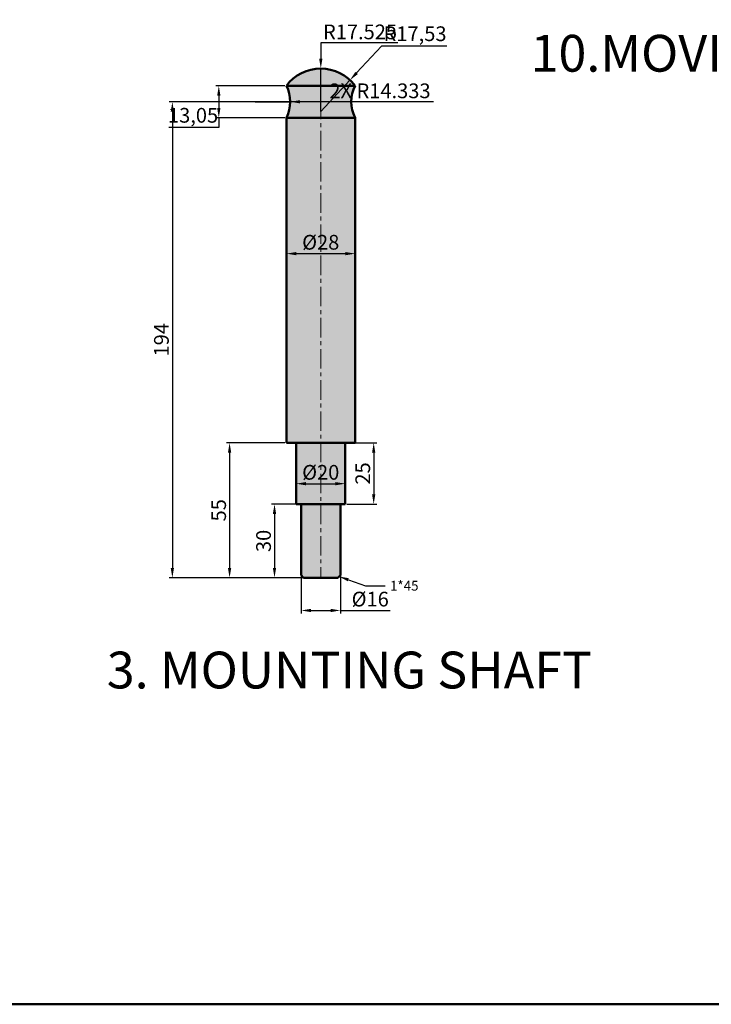
# Model space of a CAD drawing. Units: millimetres. Extents: x -14 to 1073, y -445 to 318.
# Tile 2 of 6: x 415 to 697, y -445 to -44. Entities that reach past the tile are written whole.
import ezdxf
from ezdxf import colors
from ezdxf.entities.mleader import LeaderData, LeaderLine
from ezdxf.math import Vec2, Vec3

# ---------------------------------------------------------------- set-up
doc = ezdxf.new("R2010")
doc.units = ezdxf.units.MM
doc.header["$LTSCALE"] = 0.5
doc.linetypes.add('CENTER', pattern=[50.8, 31.75, -6.35, 6.35, -6.35])
doc.linetypes.add('HIDDEN', pattern=[9.525, 6.35, -3.175])
for name, color, linetype, lineweight in [('M-CNTR', 1, 'CENTER', 18), ('M-DIMS', 2, 'Continuous', 25), ('M-HATC', 8, 'Continuous', 18), ('M-HIDN', 4, 'HIDDEN', 25), ('M-OUTL', 7, 'Continuous', 50), ('M-TEXT', 3, 'Continuous', 25)]:
    doc.layers.add(name, color=color, linetype=linetype, lineweight=lineweight)
doc.styles.get("Standard").update_dxf_attribs({"font": 'arial.ttf'})
doc.dimstyles.new('ISO-25', dxfattribs={"dimtxt": 6, "dimasz": 4, "dimexe": 1.25, "dimexo": 0.625, "dimtad": 1, "dimtoh": 1, "dimtxsty": 'Standard', "dimcen": 2.5, "dimadec": 0, "dimazin": 0, "dimtfac": 1, "dimtmove": 0, "dimatfit": 3, "dimfxl": 1, "dimarcsym": 0})

# ---------------------------------------------------------------- blocks, each defined once
blk = doc.blocks.new('*D38')
at = {"layer": 'Defpoints', "color": 0, "ltscale": 0.5, "transparency": 16777216}
for p in [(547.87, -216.31), (547.87, -241.31), (559.47, -241.31)]:
    blk.add_point(p, dxfattribs=at)
at = {"layer": 'M-DIMS', "color": 0, "lineweight": -2, "ltscale": 0.5, "transparency": 16777216}
for p, q in [((548.49, -216.31), (560.72, -216.31)), ((559.47, -220.31), (559.47, -237.31)), ((548.49, -241.31), (560.72, -241.31))]:
    blk.add_line(p, q, dxfattribs=at)
at = {"layer": 'M-DIMS', "color": 0, "ltscale": 0.5, "transparency": 16777216}
for points in [[(558.8, -220.31), (560.13, -220.31), (559.47, -216.31)], [(558.8, -237.31), (560.13, -237.31), (559.47, -241.31)]]:
    blk.add_solid(points, dxfattribs=at)
at = {"layer": 'M-DIMS', "color": 0, "ltscale": 0.5, "transparency": 16777216, "insert": (555.78, -228.81), "char_height": 6, "attachment_point": 5, "rotation": 90}
blk.add_mtext('25', dxfattribs=at)
blk = doc.blocks.new('*D39')
at = {"layer": 'Defpoints', "color": 0, "ltscale": 0.5, "transparency": 16777216}
for p in [(529.87, -241.31), (519.03, -271.31), (530.87, -271.31)]:
    blk.add_point(p, dxfattribs=at)
at = {"layer": 'M-DIMS', "color": 0, "lineweight": -2, "ltscale": 0.5, "transparency": 16777216}
for p, q in [((529.24, -241.31), (517.78, -241.31)), ((519.03, -245.31), (519.03, -267.31)), ((530.24, -271.31), (517.78, -271.31))]:
    blk.add_line(p, q, dxfattribs=at)
at = {"layer": 'M-DIMS', "color": 0, "ltscale": 0.5, "transparency": 16777216}
for points in [[(518.36, -245.31), (519.7, -245.31), (519.03, -241.31)], [(518.36, -267.31), (519.7, -267.31), (519.03, -271.31)]]:
    blk.add_solid(points, dxfattribs=at)
at = {"layer": 'M-DIMS', "color": 0, "ltscale": 0.5, "transparency": 16777216, "insert": (515.34, -256.31), "char_height": 6, "attachment_point": 5, "rotation": 90}
blk.add_mtext('30', dxfattribs=at)
blk = doc.blocks.new('*D40')
at = {"layer": 'Defpoints', "color": 0, "ltscale": 0.5, "transparency": 16777216}
for p in [(523.87, -216.31), (500.71, -271.31), (529.87, -271.31)]:
    blk.add_point(p, dxfattribs=at)
at = {"layer": 'M-DIMS', "color": 0, "lineweight": -2, "ltscale": 0.5, "transparency": 16777216}
for p, q in [((523.24, -216.31), (499.46, -216.31)), ((500.71, -220.31), (500.71, -267.31)), ((529.24, -271.31), (499.46, -271.31))]:
    blk.add_line(p, q, dxfattribs=at)
at = {"layer": 'M-DIMS', "color": 0, "ltscale": 0.5, "transparency": 16777216}
for points in [[(500.04, -220.31), (501.38, -220.31), (500.71, -216.31)], [(500.04, -267.31), (501.38, -267.31), (500.71, -271.31)]]:
    blk.add_solid(points, dxfattribs=at)
at = {"layer": 'M-DIMS', "color": 0, "ltscale": 0.5, "transparency": 16777216, "insert": (497.03, -243.81), "char_height": 6, "attachment_point": 5, "rotation": 90}
blk.add_mtext('55', dxfattribs=at)
blk = doc.blocks.new('*D41')
at = {"layer": 'Defpoints', "color": 0, "ltscale": 0.5, "transparency": 16777216}
for p in [(523.87, -139.87), (551.87, -139.21), (551.87, -139.87)]:
    blk.add_point(p, dxfattribs=at)
at = {"layer": 'M-DIMS', "color": 0, "lineweight": -2, "ltscale": 0.5, "transparency": 16777216}
for p, q in [((523.87, -139.25), (523.87, -137.96)), ((527.87, -139.21), (547.87, -139.21)), ((551.87, -139.25), (551.87, -137.96))]:
    blk.add_line(p, q, dxfattribs=at)
at = {"layer": 'M-DIMS', "color": 0, "ltscale": 0.5, "transparency": 16777216}
for points in [[(527.87, -138.54), (527.87, -139.87), (523.87, -139.21)], [(547.87, -138.54), (547.87, -139.87), (551.87, -139.21)]]:
    blk.add_solid(points, dxfattribs=at)
at = {"layer": 'M-DIMS', "color": 0, "ltscale": 0.5, "transparency": 16777216, "insert": (537.87, -135.35), "char_height": 6, "attachment_point": 5}
blk.add_mtext('%%C28', dxfattribs=at)
blk = doc.blocks.new('*D42')
at = {"layer": 'Defpoints', "color": 0, "ltscale": 0.5, "transparency": 16777216}
for p in [(523.87, -70.78), (496.32, -83.83), (523.87, -83.83)]:
    blk.add_point(p, dxfattribs=at)
at = {"layer": 'M-DIMS', "color": 0, "lineweight": -2, "ltscale": 0.5, "transparency": 16777216}
for p, q in [((523.24, -70.78), (495.07, -70.78)), ((496.32, -74.78), (496.32, -79.83)), ((523.24, -83.83), (495.07, -83.83)), ((496.32, -83.83), (496.32, -87.83)), ((496.32, -87.83), (475.97, -87.83))]:
    blk.add_line(p, q, dxfattribs=at)
at = {"layer": 'M-DIMS', "color": 0, "ltscale": 0.5, "transparency": 16777216}
for points in [[(495.66, -74.78), (496.99, -74.78), (496.32, -70.78)], [(495.66, -79.83), (496.99, -79.83), (496.32, -83.83)]]:
    blk.add_solid(points, dxfattribs=at)
at = {"layer": 'M-DIMS', "color": 0, "ltscale": 0.5, "transparency": 16777216, "insert": (485.83, -83.6), "char_height": 6, "attachment_point": 5}
blk.add_mtext('13,05', dxfattribs=at)
blk = doc.blocks.new('*D43')
at = {"layer": 'Defpoints', "color": 0, "ltscale": 0.5, "transparency": 16777216}
for p in [(537.87, -77.31), (477.39, -271.31), (537.87, -271.31)]:
    blk.add_point(p, dxfattribs=at)
at = {"layer": 'M-DIMS', "color": 0, "lineweight": -2, "ltscale": 0.5, "transparency": 16777216}
for p, q in [((537.24, -77.31), (476.14, -77.31)), ((477.39, -81.31), (477.39, -267.31)), ((537.24, -271.31), (476.14, -271.31))]:
    blk.add_line(p, q, dxfattribs=at)
at = {"layer": 'M-DIMS', "color": 0, "ltscale": 0.5, "transparency": 16777216}
for points in [[(476.72, -81.31), (478.05, -81.31), (477.39, -77.31)], [(476.72, -267.31), (478.05, -267.31), (477.39, -271.31)]]:
    blk.add_solid(points, dxfattribs=at)
at = {"layer": 'M-DIMS', "color": 0, "ltscale": 0.5, "transparency": 16777216, "insert": (473.7, -174.31), "char_height": 6, "attachment_point": 5, "rotation": 90}
blk.add_mtext('194', dxfattribs=at)
blk = doc.blocks.new('*D44')
at = {"layer": 'Defpoints', "color": 0, "ltscale": 0.5, "transparency": 16777216}
for p in [(549.79, -68.49), (537.87, -81.33)]:
    blk.add_point(p, dxfattribs=at)
at = {"layer": 'M-DIMS', "color": 0, "lineweight": -2, "ltscale": 0.5, "transparency": 16777216}
for p, q in [((562.71, -54.58), (552.52, -65.55)), ((589.32, -54.58), (562.71, -54.58)), ((537.87, -81.33), (549.79, -68.49))]:
    blk.add_line(p, q, dxfattribs=at)
at = {"layer": 'M-DIMS', "color": 0, "ltscale": 0.5, "transparency": 16777216}
blk.add_solid([(552.03, -65.1), (553.01, -66.01), (549.79, -68.49)], dxfattribs=at)
at = {"layer": 'M-DIMS', "color": 0, "ltscale": 0.5, "transparency": 16777216, "insert": (576.33, -50.35), "char_height": 6, "attachment_point": 5}
blk.add_mtext('R17,53', dxfattribs=at)
blk = doc.blocks.new('*D45')
at = {"layer": 'Defpoints', "color": 0, "ltscale": 0.5, "transparency": 16777216}
for p in [(529.87, -267.73), (545.87, -267.73), (545.87, -284.65)]:
    blk.add_point(p, dxfattribs=at)
at = {"layer": 'M-DIMS', "color": 0, "lineweight": -2, "ltscale": 0.5, "transparency": 16777216}
for p, q in [((529.87, -268.36), (529.87, -285.9)), ((545.87, -268.36), (545.87, -285.9)), ((533.87, -284.65), (541.87, -284.65)), ((545.87, -284.65), (566.24, -284.65))]:
    blk.add_line(p, q, dxfattribs=at)
at = {"layer": 'M-DIMS', "color": 0, "ltscale": 0.5, "transparency": 16777216}
for points in [[(533.87, -283.98), (533.87, -285.32), (529.87, -284.65)], [(541.87, -283.98), (541.87, -285.32), (545.87, -284.65)]]:
    blk.add_solid(points, dxfattribs=at)
at = {"layer": 'M-DIMS', "color": 0, "ltscale": 0.5, "transparency": 16777216, "insert": (558.05, -280.8), "char_height": 6, "attachment_point": 5}
blk.add_mtext('%%C16', dxfattribs=at)
blk = doc.blocks.new('*D46')
at = {"layer": 'Defpoints', "color": 0, "ltscale": 0.5, "transparency": 16777216}
for p in [(527.87, -232.97), (547.87, -232.97), (547.87, -232.97)]:
    blk.add_point(p, dxfattribs=at)
at = {"layer": 'M-DIMS', "color": 0, "lineweight": -2, "ltscale": 0.5, "transparency": 16777216}
for p, q in [((527.87, -232.35), (527.87, -231.72)), ((547.87, -232.35), (547.87, -231.72)), ((531.87, -232.97), (543.87, -232.97))]:
    blk.add_line(p, q, dxfattribs=at)
at = {"layer": 'M-DIMS', "color": 0, "ltscale": 0.5, "transparency": 16777216}
for points in [[(531.87, -232.31), (531.87, -233.64), (527.87, -232.97)], [(543.87, -232.31), (543.87, -233.64), (547.87, -232.97)]]:
    blk.add_solid(points, dxfattribs=at)
at = {"layer": 'M-DIMS', "color": 0, "ltscale": 0.5, "transparency": 16777216, "insert": (537.87, -229.12), "char_height": 6, "attachment_point": 5}
blk.add_mtext('%%C20', dxfattribs=at)
blk = doc.blocks.new('*D86')
at = {"layer": 'Defpoints', "color": 0, "ltscale": 0.5, "transparency": 16777216}
for p in [(537.9, -63.8), (537.87, -81.33)]:
    blk.add_point(p, dxfattribs=at)
at = {"layer": 'M-DIMS', "color": 0, "lineweight": -2, "ltscale": 0.5, "transparency": 16777216}
for p, q in [((537.92, -53.29), (537.91, -59.8)), ((569.24, -53.29), (537.92, -53.29)), ((537.87, -81.33), (537.9, -63.8))]:
    blk.add_line(p, q, dxfattribs=at)
at = {"layer": 'M-DIMS', "color": 0, "ltscale": 0.5, "transparency": 16777216}
blk.add_solid([(537.24, -59.8), (538.57, -59.8), (537.9, -63.8)], dxfattribs=at)
at = {"layer": 'M-DIMS', "color": 0, "ltscale": 0.5, "transparency": 16777216, "insert": (553.89, -49.6), "char_height": 6, "attachment_point": 5}
blk.add_mtext('R17.525', dxfattribs=at)
blk = doc.blocks.new('*D87')
at = {"layer": 'Defpoints', "color": 0, "ltscale": 0.5, "transparency": 16777216}
for p in [(511.11, -77.31), (525.44, -77.31)]:
    blk.add_point(p, dxfattribs=at)
at = {"layer": 'M-DIMS', "color": 0, "lineweight": -2, "ltscale": 0.5, "transparency": 16777216}
for p, q in [((511.11, -77.31), (525.44, -77.31)), ((539.57, -77.31), (529.44, -77.31)), ((583.84, -77.31), (539.57, -77.31))]:
    blk.add_line(p, q, dxfattribs=at)
at = {"layer": 'M-DIMS', "color": 0, "ltscale": 0.5, "transparency": 16777216}
blk.add_solid([(529.44, -76.64), (529.44, -77.98), (525.44, -77.31)], dxfattribs=at)
at = {"layer": 'M-DIMS', "color": 0, "ltscale": 0.5, "transparency": 16777216, "insert": (562.02, -73.62), "char_height": 6, "attachment_point": 5}
blk.add_mtext('2X R14.333', dxfattribs=at)

msp = doc.modelspace()

# ---------------------------------------------------------------- hatches: boundary and pattern name
at = {"layer": 'M-HATC', "ltscale": 0.5}
h = msp.add_hatch(color=256, dxfattribs=at)
h.set_gradient(color1=(209, 156, 199), color2=(128, 128, 128), tint=1, name='CYLINDER')
h.paths.add_polyline_path([(551.8681, -83.8341), (537.8681, -83.8341), (537.8681, -216.3091), (551.8681, -216.3091)])
h.paths.add_polyline_path([(537.8681, -83.8341), (523.8681, -83.8341), (523.8681, -216.3091), (537.8681, -216.3091)])
h.paths.add_polyline_path([(537.8681, -70.7841), (523.8681, -70.7841, -0.11871814), (525.4395, -77.3091), (537.8681, -77.3091)])
h.paths.add_polyline_path([(537.8681, -77.3091), (525.4395, -77.3091, -0.11871814), (523.8681, -83.8341), (537.8681, -83.8341)])
h.paths.add_polyline_path([(550.2967, -77.3091), (537.8681, -77.3091), (537.8681, -83.8341), (551.8681, -83.8341, -0.11871814)])
h.paths.add_polyline_path([(551.8681, -70.7841), (537.8681, -70.7841), (537.8681, -77.3091), (550.2967, -77.3091, -0.11871814)])
h.paths.add_polyline_path([(537.8681, -63.8009), (537.8681, -70.7841), (551.8681, -70.7841, 0.23556007)])
h.paths.add_polyline_path([(537.8681, -63.8009, 0.23556007), (523.8681, -70.7841), (537.8681, -70.7841)])
h.paths.add_polyline_path([(547.8681, -216.3091), (537.8681, -216.3091), (537.8681, -241.3091), (547.8681, -241.3091)])
h.paths.add_polyline_path([(545.8681, -241.3091), (537.8681, -241.3091), (537.8681, -271.3091), (544.8681, -271.3091), (545.8681, -270.3091)])
h.paths.add_polyline_path([(537.8681, -241.3091), (529.8681, -241.3091), (529.8681, -270.3091), (530.8681, -271.3091), (537.8681, -271.3091)])
h.paths.add_polyline_path([(537.8681, -216.3091), (527.8681, -216.3091), (527.8681, -241.3091), (537.8681, -241.3091)])
h.paths.add_polyline_path([(531.7842, -231.358), (544.1075, -231.358), (544.1075, -218.9938), (531.7842, -218.9938)], flags=9)
h = msp.add_hatch(color=256, dxfattribs=at)
h.set_gradient(color1=(209, 156, 199), color2=(128, 128, 128), tint=1, name='CYLINDER')
h.paths.add_polyline_path([(537.8681, -216.3091), (527.8681, -216.3091), (527.8681, -241.3091), (537.8681, -241.3091)])
h.paths.add_polyline_path([(547.8681, -216.3091), (537.8681, -216.3091), (537.8681, -241.3091), (547.8681, -241.3091)])

# ---------------------------------------------------------------- linework, layer by layer
at = {"layer": 'M-CNTR', "ltscale": 0.5}
msp.add_line((537.8681, -63.8009), (537.8681, -271.3091), dxfattribs=at)
at = {"layer": 'M-HIDN', "ltscale": 0.5}
msp.add_line((550.2967, -77.3091), (525.4395, -77.3091), dxfattribs=at)
at = {"layer": 'M-OUTL', "ltscale": 0.5}
for p, q in [((551.8681, -70.7841), (523.8681, -70.7841)), ((523.8681, -83.8341), (523.8681, -216.3091)), ((551.8681, -83.8341), (523.8681, -83.8341)), ((551.8681, -83.8341), (551.8681, -216.3091)), ((523.8681, -216.3091), (551.8681, -216.3091)), ((527.8681, -216.3091), (527.8681, -241.3091)), ((547.8681, -216.3091), (547.8681, -241.3091)), ((547.8681, -241.3091), (527.8681, -241.3091)), ((529.8681, -241.3091), (529.8681, -270.3091)), ((545.8681, -270.3091), (545.8681, -241.3091)), ((529.8681, -270.3091), (530.8681, -271.3091)), ((530.8681, -271.3091), (537.8681, -271.3091)), ((537.8681, -271.3091), (544.8681, -271.3091)), ((544.8681, -271.3091), (545.8681, -270.3091))]:
    msp.add_line(p, q, dxfattribs=at)
msp.add_lwpolyline([(-13.7695, 318.0907), (1072.7514, 318.0907), (1072.7514, -445.1795), (-13.7695, -445.1795)], close=True, dxfattribs=at)
for centre, radius, start, end in [((537.8681, -81.3262), 17.5253, 36.980172, 143.01983), ((511.107, -77.3091), 14.3326, 332.91856, 27.08144), ((564.6293, -77.3091), 14.3326, 152.91856, 207.08144)]:
    msp.add_arc(centre, radius, start, end, dxfattribs=at)

# ---------------------------------------------------------------- texts
at = {"layer": 'M-TEXT', "ltscale": 0.5, "char_height": 15, "attachment_point": 1}
for s, width, insert in [('\\pxqc;10.MOVING PIN', 154.431653, (618.8169, -50.0413)), ('\\pxqc;3. MOUNTING SHAFT', 218.927832, (440.1026, -301.4245))]:
    msp.add_mtext_dynamic_manual_height_columns(s, width=width, gutter_width=12.5, heights=[0], dxfattribs=dict(at, insert=insert))

# ---------------------------------------------------------------- dimensions: what is measured, and where the dimension line sits
at = {"layer": 'M-DIMS', "ltscale": 0.5}
for mpoint, override, picture, middle in [((537.9, -63.8009), {"dimdec": 3, "dimlfac": 1, "dimrnd": 0, "dimzin": 0, "dimdsep": 46, "dimlunit": 2}, '*D86', (553.892, -53.2858)), ((549.7949, -68.4853), {"dimclrd": 0, "dimclre": 0, "dimclrt": 0}, '*D44', (576.3264, -54.5836))]:
    dim = msp.add_radius_dim(center=(537.8681, -81.3262), mpoint=mpoint, dimstyle='ISO-25', override=override, dxfattribs=at)
    dim.commit()
    dim.dimension.update_dxf_attribs({"geometry": picture, "text_midpoint": middle, "dimtype": 164})
dim = msp.add_radius_dim(center=(511.107, -77.3091), mpoint=(525.4395, -77.31), text='2X <>', dimstyle='ISO-25', override={"dimdec": 3, "dimlfac": 1, "dimrnd": 0, "dimzin": 0, "dimdsep": 46, "dimlunit": 2}, dxfattribs=at)
dim.commit()
dim.dimension.update_dxf_attribs({"geometry": '*D87', "text_midpoint": (562.0182, -73.6204)})
for base, p1, p2, picture, middle in [((496.3231, -83.8341), (523.8681, -70.7841), (523.8681, -83.8341), '*D42', (485.8345, -83.6033)), ((477.3883, -271.3091), (537.8681, -77.3091), (537.8681, -271.3091), '*D43', (473.6999, -174.3091)), ((500.71, -271.3091), (523.8681, -216.3091), (529.8681, -271.3091), '*D40', (497.0338, -243.8091)), ((559.4677, -241.3091), (547.8681, -216.3091), (547.8681, -241.3091), '*D38', (555.7793, -228.8091)), ((519.0309, -271.3091), (529.8681, -241.3091), (530.8681, -271.3091), '*D39', (515.3404, -256.3091))]:
    dim = msp.add_linear_dim(base=base, p1=p1, p2=p2, angle=90, dimstyle='ISO-25', override={"dimclrd": 0, "dimclre": 0, "dimclrt": 0}, dxfattribs=at)
    dim.commit()
    dim.dimension.update_dxf_attribs({"geometry": picture, "text_midpoint": middle})
dim = msp.add_linear_dim(base=(551.8681, -139.2059), p1=(523.8681, -139.8743), p2=(551.8681, -139.8743), text='%%C<>', dimstyle='ISO-25', override={"dimclrd": 0, "dimclre": 0, "dimclrt": 0}, dxfattribs=at)
dim.commit()
dim.dimension.update_dxf_attribs({"geometry": '*D41', "text_midpoint": (537.8681, -139.2059), "dimtype": 160})
for base, p1, p2, picture, middle in [((547.8681, -232.9748), (527.8681, -232.9748), (547.8681, -232.9748), '*D46', (537.8681, -229.1186)), ((545.8681, -284.6516), (529.8681, -267.7309), (545.8681, -267.7309), '*D45', (558.0525, -280.7953))]:
    dim = msp.add_linear_dim(base=base, p1=p1, p2=p2, text='%%C<>', dimstyle='ISO-25', override={"dimclrd": 0, "dimclre": 0, "dimclrt": 0}, dxfattribs=at)
    dim.commit()
    dim.dimension.update_dxf_attribs({"geometry": picture, "text_midpoint": middle})

# ---------------------------------------------------------------- leaders
ml = msp.add_multileader_mtext('Standard', dxfattribs=at)
ml.set_content('1*45', color=256)
ml.set_leader_properties()
ml.build(insert=Vec2(0, 0))
ctx = ml.context
ctx.base_point, ctx.plane_origin = Vec3(564.1154, -274.5986), Vec3(545.3681, -270.8091)
notes = []
notes.append((ctx, [(0, (1, 1, 0), (556.1154, -274.5986), (1, 0), 8, [(0, [(545.3681, -270.8091)], 0, [])])]))
ctx.mtext.insert, ctx.mtext.flow_direction = Vec3(566.1154, -272.5645), 5
for ctx, leaders in notes:
    for number, flags, end, landing, length, lines in leaders:
        leader = LeaderData()
        leader.index, (leader.has_last_leader_line, leader.has_dogleg_vector, leader.attachment_direction) = number, flags
        leader.last_leader_point, leader.dogleg_vector, leader.dogleg_length = Vec3(end), Vec3(landing), length
        for number, points, colour, breaks in lines:
            line = LeaderLine()
            line.index, line.vertices, line.color, line.breaks = number, Vec3.list(points), colors.encode_raw_color(colour), breaks
            leader.lines.append(line)
        ctx.leaders.append(leader)

doc.saveas('drawing.dxf')
